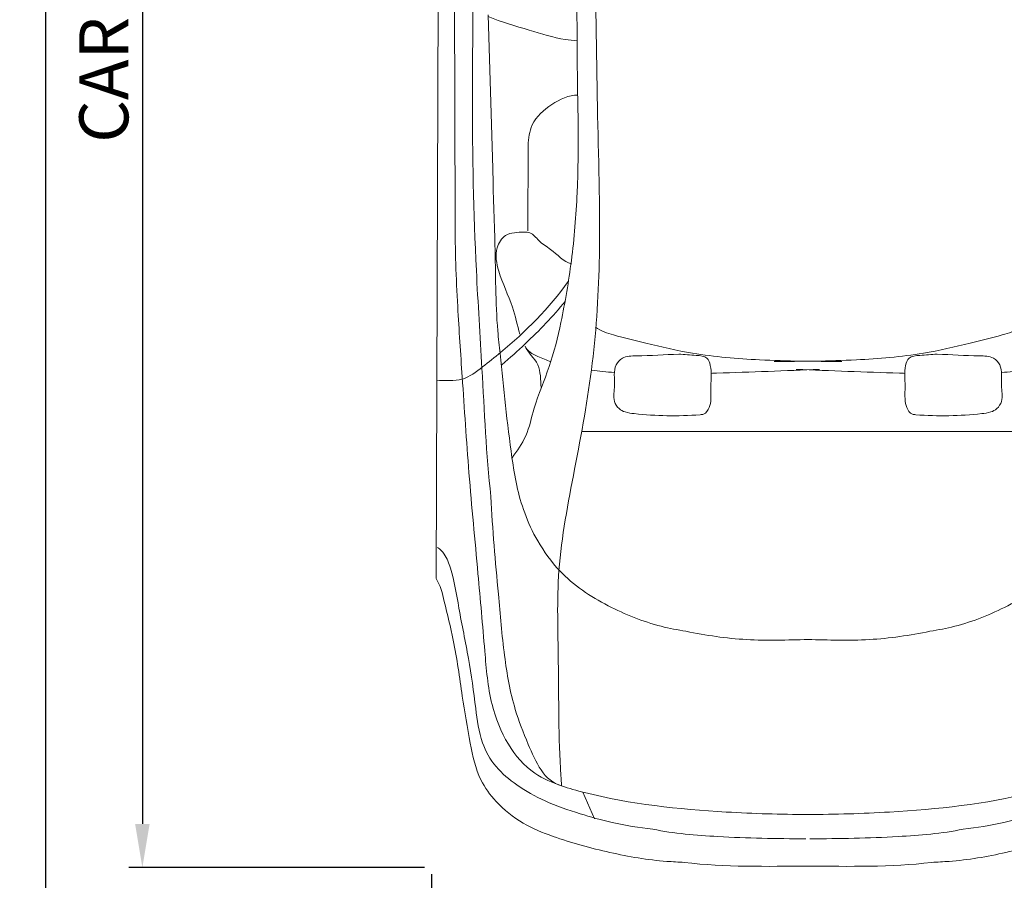
# Model space of a CAD drawing. Units: inches. Extents: x 1239 to 2276906, y 2273 to 321338.
# Tile 8 of 23: x 1664 to 1754, y 2428 to 2507. Entities that reach past the tile are written whole.
import ezdxf

# ---------------------------------------------------------------- set-up
doc = ezdxf.new("R2010")
doc.units = ezdxf.units.IN
doc.layers.add('A-ANNO-DIMS', color=2, linetype='Continuous', lineweight=18)
doc.layers.add('C-PRKG', color=8, linetype='Continuous', lineweight=13)
doc.styles.get("Standard").update_dxf_attribs({"font": 'arial.ttf'})
doc.dimstyles.new('ISO-25', dxfattribs={"dimtxt": 4.5, "dimasz": 4, "dimexe": 1.25, "dimexo": 0.625, "dimtad": 1, "dimdec": 1, "dimlunit": 3, "dimtxsty": 'Standard', "dimcen": 2.5, "dimadec": 0, "dimazin": 0, "dimtfac": 1, "dimtdec": 1, "dimtmove": 0, "dimatfit": 3, "dimfxl": 1, "dimarcsym": 0})

# ---------------------------------------------------------------- blocks, each defined once
blk = doc.blocks.new('A$C242571DA')
for p, q in [((3474.6, 1401.1), (3474.6, 843)), ((3474.6, 345.6), (3474.6, 903.8)), ((4315.2, 348.7), (4377.3, 376.3)), ((3007.2, 220.3), (2808.1, 221.6)), ((2503.3, 128.2), (2861.6, 139.2)), ((1681.8, 95.1), (2695.2, 91.4)), ((1699.9, 47.3), (2984.7, 51)), ((1714.3, 14.2), (3817.1, 6.9))]:
    blk.add_line(p, q)
for points, knots in [([(3745.3, 1736.8), (3748.5, 1730.1), (3764.2, 1717.1), (3811.5, 1698.6), (3894.7, 1686.7), (4002.9, 1663.2), (4107.9, 1648.7), (4195.8, 1638.3), (4258.6, 1603.2), (4302.1, 1549.7), (4339.9, 1483.8), (4365.2, 1407.6), (4389.6, 1324.4), (4397.9, 1266.9), (4401.8, 1235.2)], [0, 0, 0, 0, 0.0219205, 0.0572122, 0.1522539, 0.2718866, 0.3894011, 0.4710097, 0.5346344, 0.5986698, 0.6733118, 0.758696, 0.8351341, 0.9293726, 0.9293726, 0.9293726, 0.9293726]), ([(3817.1, 1739.9), (3833.2, 1729.7), (3882.9, 1718.2), (3973.3, 1695.2), (4085.1, 1680.5), (4193.8, 1662.8), (4280.6, 1644.3), (4343.9, 1598.1), (4390, 1540.3), (4427.4, 1448.7), (4457.8, 1336.6), (4475.7, 1233.4), (4478.4, 1175.1), (4479.3, 1161.6)], [0, 0, 0, 0, 0.056668, 0.14946, 0.28161, 0.392935, 0.481686, 0.542967, 0.622845, 0.69797, 0.833643, 0.965665, 1.00577, 1.00577, 1.00577, 1.00577]), ([(2984.7, 1695.8), (3051, 1695.6), (3172.1, 1691.3), (3367.4, 1677.6), (3575.2, 1664.3), (3788.2, 1643.6), (3968, 1628.1), (4103.8, 1616.8), (4203.6, 1578.1), (4271.8, 1519.5), (4300.6, 1452.1), (4341.7, 1305.3), (4361.8, 1111.2), (4367.5, 936.8), (4367.5, 873.4)], [0, 0, 0, 0, 0.198873, 0.363323, 0.587433, 0.823543, 1.004622, 1.129816, 1.230113, 1.320655, 1.388577, 1.443334, 1.771447, 1.958652, 1.958652, 1.958652, 1.958652]), ([(3664.1, 1533.3), (3687, 1526), (3734.8, 1502.3), (3816.7, 1444.8), (3884.1, 1342.9), (3925.1, 1239.9), (3937.3, 1177), (3940.4, 1157.6)], [0, 0, 0, 0, 0.0720749, 0.1581284, 0.2958089, 0.4262456, 0.4842292, 0.4842292, 0.4842292, 0.4842292]), ([(3231.5, 1368.3), (3240.8, 1356.2), (3253.1, 1315.7), (3271.9, 1240.7), (3297.9, 1127.9), (3310.5, 974.6), (3311.2, 858.3), (3311.6, 794.4)], [0, 0, 0, 0, 0.0451009, 0.1211996, 0.2308505, 0.385263, 0.5739042, 0.5739042, 0.5739042, 0.5739042]), ([(3294.8, 1174.5), (3294.8, 1207.4), (3299.6, 1249.5), (3298.3, 1303.9), (3326.3, 1329), (3363.9, 1320.7), (3399.3, 1329.3), (3422.1, 1315.7), (3430.7, 1297.9), (3438.7, 1234.2), (3439.6, 1174.4), (3434.7, 1112.2), (3418.9, 1102), (3395.9, 1098.6), (3362.6, 1100.9), (3331.1, 1096.6), (3298.8, 1107.6), (3297.3, 1140.3), (3294.8, 1160.9), (3294.8, 1174.5)], [0, 0, 0, 0, 0.0969044, 0.1295913, 0.1506192, 0.1985921, 0.2360698, 0.2557908, 0.2719711, 0.2929882, 0.44406, 0.4519132, 0.4720918, 0.4918599, 0.5228758, 0.5707096, 0.5892096, 0.6145759, 0.654681, 0.654681, 0.654681, 0.654681]), ([(4401.8, 1235.2), (4411.9, 1185.3), (4421.6, 1065.8), (4424.1, 946.5), (4424.1, 878)], [0, 0, 0, 0, 0.1502861, 0.3522699, 0.3522699, 0.3522699, 0.3522699]), ([(3940.4, 1157.6), (3949.9, 1111), (3964.3, 1016.4), (3960.5, 921), (3959.8, 873.4)], [0, 0, 0, 0, 0.140379, 0.2808468, 0.2808468, 0.2808468, 0.2808468]), ([(3339.2, 1099), (3339.1, 1094.8), (3336.4, 1010.6), (3333.2, 926.3), (3330, 846.2)], [11.235438, 11.235438, 11.235438, 11.235438, 11.552536, 17.586883, 17.586883, 17.586883, 17.586883]), ([(3231.5, 378.5), (3240.8, 390.5), (3253.1, 431), (3271.9, 506.1), (3297.9, 618.9), (3310.5, 772.1), (3311.2, 888.4), (3311.6, 952.4)], [0, 0, 0, 0, 0.0451009, 0.1211996, 0.2308505, 0.385263, 0.5739042, 0.5739042, 0.5739042, 0.5739042]), ([(3339.2, 647.8), (3339.1, 652), (3336.4, 736.2), (3333.2, 820.5), (3330, 900.6)], [11.235438, 11.235438, 11.235438, 11.235438, 11.552536, 17.586883, 17.586883, 17.586883, 17.586883]), ([(2984.7, 51), (3051, 51.1), (3172.1, 55.5), (3367.4, 69.2), (3575.2, 82.5), (3788.2, 103.1), (3968, 118.7), (4103.8, 130), (4203.6, 168.6), (4271.8, 227.3), (4300.6, 294.7), (4341.7, 441.5), (4361.8, 635.5), (4367.5, 809.9), (4367.5, 873.4)], [0, 0, 0, 0, 0.198873, 0.363323, 0.587433, 0.823543, 1.004622, 1.129816, 1.230113, 1.320655, 1.388577, 1.443334, 1.771447, 1.958652, 1.958652, 1.958652, 1.958652]), ([(3940.4, 589.1), (3949.9, 635.7), (3964.3, 730.4), (3960.5, 825.8), (3959.8, 873.4)], [0, 0, 0, 0, 0.140379, 0.2808468, 0.2808468, 0.2808468, 0.2808468]), ([(4401.8, 511.5), (4411.9, 561.5), (4421.6, 681), (4424.1, 800.3), (4424.1, 868.8)], [0, 0, 0, 0, 0.1502861, 0.3522699, 0.3522699, 0.3522699, 0.3522699]), ([(3294.8, 572.3), (3294.8, 539.4), (3299.6, 497.2), (3298.3, 442.9), (3326.3, 417.8), (3363.9, 426), (3399.3, 417.5), (3422.1, 431), (3430.7, 448.9), (3438.7, 512.5), (3439.6, 572.4), (3434.7, 634.6), (3418.9, 644.7), (3395.9, 648.2), (3362.6, 645.9), (3331.1, 650.1), (3298.8, 639.2), (3297.3, 606.5), (3294.8, 585.9), (3294.8, 572.3)], [0, 0, 0, 0, 0.0969044, 0.1295913, 0.1506192, 0.1985921, 0.2360698, 0.2557908, 0.2719711, 0.2929882, 0.44406, 0.4519132, 0.4720918, 0.4918599, 0.5228758, 0.5707096, 0.5892096, 0.6145759, 0.654681, 0.654681, 0.654681, 0.654681]), ([(3664.1, 213.5), (3687, 220.8), (3734.8, 244.4), (3816.7, 302), (3884.1, 403.8), (3925.1, 506.9), (3937.3, 569.7), (3940.4, 589.1)], [0, 0, 0, 0, 0.0720749, 0.1581284, 0.2958089, 0.4262456, 0.4842292, 0.4842292, 0.4842292, 0.4842292]), ([(3817.1, 6.9), (3833.2, 17), (3882.9, 28.6), (3973.3, 51.5), (4085.1, 66.3), (4193.8, 84), (4280.6, 102.4), (4343.9, 148.6), (4390, 206.4), (4427.4, 298), (4457.8, 410.1), (4475.7, 513.3), (4478.4, 571.6), (4479.3, 585.2)], [0, 0, 0, 0, 0.056668, 0.14946, 0.28161, 0.392935, 0.481686, 0.542967, 0.622845, 0.69797, 0.833643, 0.965665, 1.00577, 1.00577, 1.00577, 1.00577]), ([(3745.3, 10), (3748.5, 16.7), (3764.2, 29.7), (3811.5, 48.1), (3894.7, 60.1), (4002.9, 83.6), (4107.9, 98), (4195.8, 108.4), (4258.6, 143.5), (4302.1, 197), (4339.9, 262.9), (4365.2, 339.2), (4389.6, 422.4), (4397.9, 479.8), (4401.8, 511.5)], [0, 0, 0, 0, 0.0219205, 0.0572122, 0.1522539, 0.2718866, 0.3894011, 0.4710097, 0.5346344, 0.5986698, 0.6733118, 0.758696, 0.8351341, 0.9293726, 0.9293726, 0.9293726, 0.9293726]), ([(1909.8, 321.9), (1933.5, 328.1), (1995.6, 339.2), (2094.4, 361), (2211.8, 369.6), (2419, 379.8), (2704.7, 380.3), (3032.7, 392.6), (3316.2, 375.8), (3558.7, 330.9), (3789.1, 285.1), (4028.9, 293.9), (4196.2, 291.5), (4292.7, 298.8), (4300.7, 299.2)], [0, 0, 0, 0, 0.073325, 0.188896, 0.303039, 0.425821, 0.811242, 1.159737, 1.41058, 1.660623, 1.899627, 2.11145, 2.377727, 2.401703, 2.401703, 2.401703, 2.401703]), ([(3535.9, 183.7), (3520.1, 195.9), (3484.4, 220.6), (3408.2, 235.8), (3323.4, 273.7), (3207.9, 301.8), (3072.6, 324.6), (2866.9, 342.1), (2626.4, 333.8), (2396.7, 335.9), (2200.9, 329.9), (2001.3, 308.6), (1732.1, 220.8), (1527.9, 167.8), (1407.5, 136)], [0, 0, 0, 0, 0.05975, 0.126928, 0.230034, 0.336675, 0.482225, 0.641324, 0.954906, 1.203173, 1.330375, 1.542773, 1.802261, 2.175545, 2.175545, 2.175545, 2.175545]), ([(2507.7, 128.3), (2521, 159.1), (2536.6, 219.7), (2559.6, 288.3), (2563.3, 326.1), (2563.8, 335.3)], [0, 0, 0, 0, 2.528586, 4.711885, 5.408215, 5.408215, 5.408215, 5.408215]), ([(2808.1, 221.6), (2791.9, 221.6), (2751.9, 227.1), (2710.6, 274.2), (2690, 315.7), (2690.5, 337.1)], [0, 0, 0, 0, 0.0486628, 0.1144515, 0.1777721, 0.1777721, 0.1777721, 0.1777721]), ([(3248.1, 201.6), (3226.9, 196.3), (3176.1, 184.7), (3113.7, 153.8), (3052.6, 141.4), (3010.4, 168), (3010.3, 201.5), (3010.3, 230.9), (3033.7, 246.6), (3052.6, 281.6), (3078.9, 303.2), (3084, 322.4)], [0, 0, 0, 0, 0.0655106, 0.1550445, 0.2094604, 0.2438604, 0.287164, 0.3001388, 0.3275984, 0.3616951, 0.4200969, 0.4200969, 0.4200969, 0.4200969]), ([(3356.5, 7.4), (3354.9, 27.5), (3360.8, 68.5), (3324, 115.2), (3255.4, 202.5), (3187.1, 270.5), (3125.2, 314.6)], [0, 0, 0, 0, 0.0597371, 0.1139981, 0.1672498, 0.3938869, 0.3938869, 0.3938869, 0.3938869]), ([(3319, 159.7), (3303.3, 178.6), (3256.9, 230), (3206.7, 279.5), (3171.4, 307.2)], [0, 0, 0, 0, 1.868162, 5.271297, 5.271297, 5.271297, 5.271297]), ([(3626.6, 134.7), (3702.5, 137.7), (3826.2, 149.9), (3991.4, 163.5), (4111.7, 184.4), (4212.2, 224.1), (4290.4, 258.8), (4300.7, 299.2)], [0, 0, 0, 0, 0.2277977, 0.3719478, 0.4996814, 0.5863441, 0.709615, 0.709615, 0.709615, 0.709615]), ([(3275.5, 214), (3287.5, 218.5), (3299.8, 241.9), (3308.4, 264.3), (3311.7, 274.2)], [0, 0, 0, 0, 0.983949, 1.771691, 1.771691, 1.771691, 1.771691]), ([(3372.2, 251.5), (3354.4, 249.9), (3316, 252), (3291.6, 220.9), (3275.5, 214)], [0, 0, 0, 0, 0.0535488, 0.1060573, 0.1060573, 0.1060573, 0.1060573]), ([(2861.6, 139.2), (2921.1, 139.4), (3047.2, 146), (3191.4, 144.8), (3356.6, 162.6), (3498.3, 176.1), (3623.2, 197.4), (3664.1, 213.5)], [0, 0, 0, 0, 0.1783018, 0.3787173, 0.431954, 0.6762374, 0.8077184, 0.8077184, 0.8077184, 0.8077184]), ([(2695.2, 91.4), (2829.9, 91.5), (3041.2, 95.4), (3351.3, 116.1), (3527.5, 123.5), (3626.6, 134.7)], [0, 0, 0, 0, 0.4042759, 0.6333827, 0.9326252, 0.9326252, 0.9326252, 0.9326252])]:
    blk.add_open_spline(points, degree=3, knots=knots)
for points in [[(3331.9, 1378.1), (3334.2, 1360.4), (3335.9, 1342.5), (3337.3, 1324.5)], [(4479.3, 1161.6), (4491, 1066.2), (4488, 969.5), (4488, 873.4)], [(4479.3, 585.2), (4491, 680.6), (4488, 777.3), (4488, 873.4)], [(3331.9, 368.6), (3334.2, 386.4), (3335.9, 404.3), (3337.3, 422.2)]]:
    blk.add_open_spline(points, degree=3)
blk = doc.blocks.new('*D58')
at = {"layer": 'A-ANNO-DIMS', "color": 0, "lineweight": -2, "transparency": 16777216}
for p, q in [((1701.17, 2606.313), (1674.023, 2606.313)), ((1675.273, 2602.313), (1675.273, 2433.5)), ((1701.17, 2429.5), (1674.023, 2429.5))]:
    blk.add_line(p, q, dxfattribs=at)
at = {"layer": 'A-ANNO-DIMS', "color": 0, "transparency": 16777216}
for points in [[(1674.607, 2602.313), (1675.94, 2602.313), (1675.273, 2606.313)], [(1674.607, 2433.5), (1675.94, 2433.5), (1675.273, 2429.5)]]:
    blk.add_solid(points, dxfattribs=at)
at = {"layer": 'Defpoints', "color": 0, "transparency": 16777216}
for p in [(1701.795, 2606.313), (1675.273, 2429.5), (1701.795, 2429.5)]:
    blk.add_point(p, dxfattribs=at)
at = {"layer": 'A-ANNO-DIMS', "color": 0, "transparency": 16777216, "insert": (1672.322, 2517.907), "char_height": 4.5, "attachment_point": 5, "rotation": 90}
blk.add_mtext('CAR 14\'-9" TYP.', dxfattribs=at)
blk = doc.blocks.new('*D59')
at = {"layer": 'A-ANNO-DIMS', "color": 0, "lineweight": -2, "transparency": 16777216}
for p, q in [((1701.795, 2428.875), (1701.795, 2401.728)), ((1770.889, 2428.875), (1770.889, 2401.728)), ((1705.795, 2402.978), (1766.889, 2402.978))]:
    blk.add_line(p, q, dxfattribs=at)
at = {"layer": 'A-ANNO-DIMS', "color": 0, "transparency": 16777216}
for points in [[(1705.795, 2403.645), (1705.795, 2402.312), (1701.795, 2402.978)], [(1766.889, 2403.645), (1766.889, 2402.312), (1770.889, 2402.978)]]:
    blk.add_solid(points, dxfattribs=at)
at = {"layer": 'Defpoints', "color": 0, "transparency": 16777216}
for p in [(1701.795, 2429.5), (1770.889, 2429.5), (1770.889, 2402.978)]:
    blk.add_point(p, dxfattribs=at)
at = {"layer": 'A-ANNO-DIMS', "color": 0, "transparency": 16777216, "insert": (1736.342, 2405.901), "char_height": 4.5, "attachment_point": 5}
blk.add_mtext('5\'-9" TYP.', dxfattribs=at)
blk = doc.blocks.new('*D87')
at = {"layer": 'A-ANNO-DIMS', "color": 0, "lineweight": -2, "transparency": 16777216}
for p, q in [((1666.383, 3250.772), (1666.383, 2275.696)), ((1921.383, 3250.772), (1921.383, 2275.696)), ((1670.383, 2276.946), (1917.383, 2276.946))]:
    blk.add_line(p, q, dxfattribs=at)
at = {"layer": 'A-ANNO-DIMS', "color": 0, "transparency": 16777216}
for points in [[(1670.383, 2277.613), (1670.383, 2276.279), (1666.383, 2276.946)], [(1917.383, 2277.613), (1917.383, 2276.279), (1921.383, 2276.946)]]:
    blk.add_solid(points, dxfattribs=at)
at = {"layer": 'Defpoints', "color": 0, "transparency": 16777216}
for p in [(1666.383, 3251.397), (1921.383, 3251.397), (1921.383, 2276.946)]:
    blk.add_point(p, dxfattribs=at)
at = {"layer": 'A-ANNO-DIMS', "color": 0, "transparency": 16777216, "insert": (1793.883, 2279.87), "char_height": 4.5, "attachment_point": 5}
blk.add_mtext('21\'-3"', dxfattribs=at)

msp = doc.modelspace()

# ---------------------------------------------------------------- block references
at = {"layer": 'C-PRKG', "xscale": 0.0393700787401575, "yscale": 0.0393700787401575, "zscale": 0.0393700787401575, "rotation": 269.9999983053478}
msp.add_blockref('A$C242571DA', (1701.957, 2606.313), dxfattribs=at)

# ---------------------------------------------------------------- dimensions: what is measured, and where the dimension line sits
at = {"layer": 'A-ANNO-DIMS'}
dim = msp.add_linear_dim(base=(1921.383, 2276.946), p1=(1666.383, 3251.397), p2=(1921.383, 3251.397), dimstyle='ISO-25', override={"dimdec": 1, "dimlfac": 1, "dimrnd": 0, "dimzin": 1, "dimdsep": 46, "dimlunit": 4, "dimfrac": 2}, dxfattribs=at)
dim.commit()
dim.dimension.update_dxf_attribs({"geometry": '*D87', "text_midpoint": (1793.883, 2279.87)})
for base, p1, p2, angle, text, picture, middle in [((1675.273, 2429.5), (1701.795, 2606.313), (1701.795, 2429.5), 270, 'CAR <> TYP.', '*D58', (1672.322, 2517.907)), ((1770.889, 2402.978), (1701.795, 2429.5), (1770.889, 2429.5), 360, '<> TYP.', '*D59', (1736.342, 2405.901))]:
    dim = msp.add_linear_dim(base=base, p1=p1, p2=p2, angle=angle, text=text, dimstyle='ISO-25', override={"dimdec": 1, "dimlfac": 1, "dimrnd": 0, "dimzin": 1, "dimdsep": 46, "dimlunit": 4, "dimfrac": 2}, dxfattribs=at)
    dim.commit()
    dim.dimension.update_dxf_attribs({"geometry": picture, "text_midpoint": middle})

doc.saveas('drawing.dxf')
